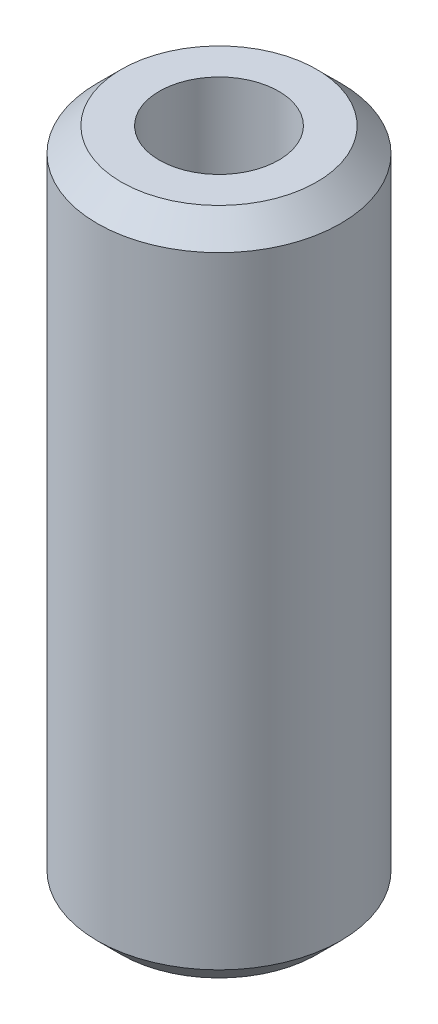
from build123d import *

# Parameters (mm, degrees)
PIN_PROFILE_25_4_12_47_R   = 12.7
PIN_PROFILE_25_4_12_47_R_2 = 6.235
PIN_BODY_69_85_DEPTH       = 34.925
END_CHAMFERS_2_5X45_SIZE   = 2.5


with BuildPart() as part:
    # Pin Profile Ø25.4-Ø12.47 → Pin Body 69.85 (new, symmetric)
    with BuildSketch(Plane(origin=(0, 0, 0), x_dir=(1, 0, 0), z_dir=(0, 1, 0))):
        with Locations(Location((0, 0, 0), (0, 0, 270))):
            Circle(PIN_PROFILE_25_4_12_47_R)
        with Locations(Location((0, 0, 0), (0, 0, 270))):
            Circle(PIN_PROFILE_25_4_12_47_R_2, mode=Mode.SUBTRACT)
    extrude(amount=PIN_BODY_69_85_DEPTH, both=True)

    # End Chamfers 2.5x45°
    end_chamfers_2_5x45_edges = [part.edges().sort_by_distance(p)[0] for p in [
        (0, -34.925, -12.7),
        (0, 34.925, -12.7),
    ]]
    chamfer(end_chamfers_2_5x45_edges, length=END_CHAMFERS_2_5X45_SIZE)


solid = part.part
